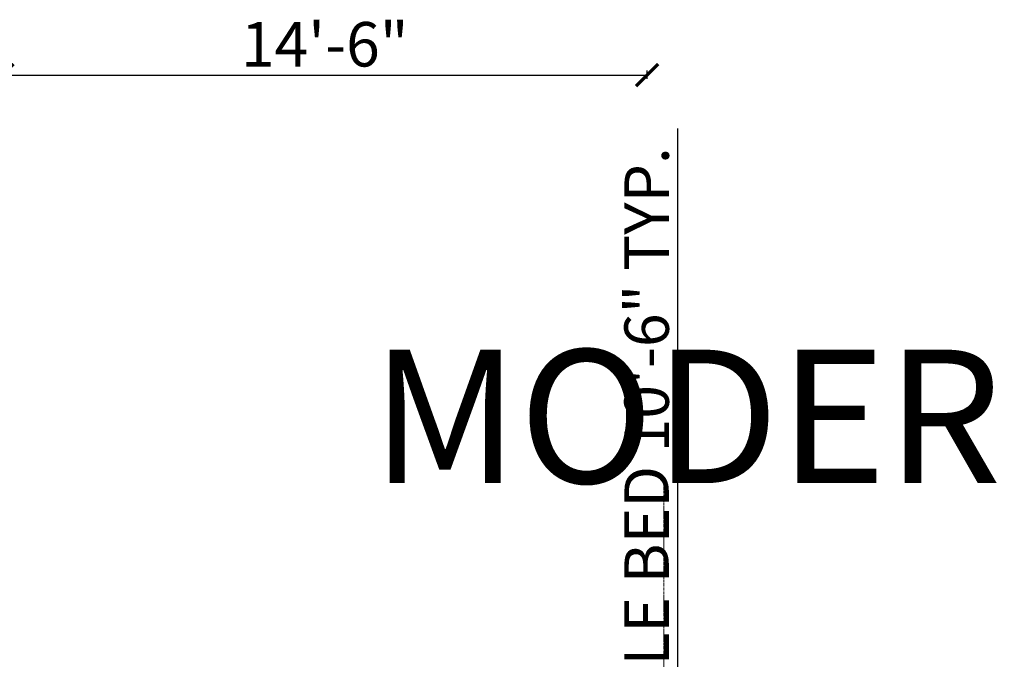
# Model space of a CAD drawing. Units: inches. Extents: x 261 to 2725, y 291 to 1454.
# Tile 16 of 35: x 777 to 1043, y 1281 to 1454. Entities that reach past the tile are written whole.
import ezdxf

# ---------------------------------------------------------------- set-up
doc = ezdxf.new("R2010")
doc.units = ezdxf.units.IN
doc.linetypes.add('CENTER', pattern=[2, 1.25, -0.25, 0.25, -0.25])
for name, color, linetype, lineweight in [('A-ANNO-DIMS', 136, 'Continuous', 18), ('A-ANNO-TEXT', 7, 'Continuous', 25), ('A-GRID', 251, 'CENTER', 13)]:
    doc.layers.add(name, color=color, linetype=linetype, lineweight=lineweight)
doc.styles.get("Standard").update_dxf_attribs({"font": 'arial.ttf'})
doc.dimstyles.new('ISO-25', dxfattribs={"dimtxt": 12, "dimasz": 6, "dimexe": 1.25, "dimexo": 0.625, "dimtad": 1, "dimdec": 0, "dimlunit": 3, "dimtxsty": 'Standard', "dimblk": 'ARCHTICK', "dimcen": 2.5, "dimadec": 0, "dimazin": 0, "dimtfac": 1, "dimtdec": 0, "dimtmove": 0, "dimatfit": 3, "dimfxl": 1, "dimfxlon": 1, "dimarcsym": 0})

# ---------------------------------------------------------------- blocks, each defined once
blk = doc.blocks.new('_ArchTick')
at = {"color": 0, "linetype": 'ByBlock', "const_width": 0.15}
blk.add_lwpolyline([(-0.5, -0.5), (0.5, 0.5)], dxfattribs=at)
blk = doc.blocks.new('*D41')
at = {"layer": 'A-ANNO-DIMS', "color": 0, "lineweight": -2, "ltscale": 0.07, "transparency": 16777216}
for p, q in [((954.74, 1222.47), (954.74, 1424.31)), ((953.74, 1222.47), (955.99, 1222.47)), ((954.74, 1096.37), (954.74, 1222.47)), ((953.74, 1096.37), (955.99, 1096.37))]:
    blk.add_line(p, q, dxfattribs=at)
at = {"layer": 'Defpoints', "color": 0, "ltscale": 0.07, "transparency": 16777216}
for p in [(935.82, 1222.47), (954.74, 1222.47), (935.82, 1096.37)]:
    blk.add_point(p, dxfattribs=at)
at = {"layer": 'A-ANNO-DIMS', "color": 0, "lineweight": -2, "ltscale": 0.07, "transparency": 16777216, "xscale": 6, "yscale": 6, "zscale": 6}
for p, rotation in [((954.74, 1222.47), 90), ((954.74, 1096.37), 270)]:
    blk.add_blockref('_ArchTick', p, dxfattribs=dict(at, rotation=rotation))
at = {"layer": 'A-ANNO-DIMS', "color": 0, "ltscale": 0.07, "transparency": 16777216, "insert": (947.9, 1326.39), "char_height": 12, "attachment_point": 5, "rotation": 90}
blk.add_mtext('DOUBLE BED 10\'-6" TYP.', dxfattribs=at)
blk = doc.blocks.new('*D76')
at = {"layer": 'A-ANNO-DIMS', "color": 0, "lineweight": -2, "ltscale": 0.07, "transparency": 16777216}
for p, q in [((772.45, 1437.76), (772.45, 1440.01)), ((772.45, 1438.76), (946.45, 1438.76)), ((946.45, 1437.76), (946.45, 1440.01))]:
    blk.add_line(p, q, dxfattribs=at)
at = {"layer": 'Defpoints', "color": 0, "ltscale": 0.07, "transparency": 16777216}
for p in [(946.45, 1438.76), (772.45, 1222.47), (946.45, 1222.47)]:
    blk.add_point(p, dxfattribs=at)
at = {"layer": 'A-ANNO-DIMS', "color": 0, "lineweight": -2, "ltscale": 0.07, "transparency": 16777216, "xscale": 6, "yscale": 6, "zscale": 6, "rotation": 180}
blk.add_blockref('_ArchTick', (772.45, 1438.76), dxfattribs=at)
at = {"layer": 'A-ANNO-DIMS', "color": 0, "lineweight": -2, "ltscale": 0.07, "transparency": 16777216, "xscale": 6, "yscale": 6, "zscale": 6}
blk.add_blockref('_ArchTick', (946.45, 1438.76), dxfattribs=at)
at = {"layer": 'A-ANNO-DIMS', "color": 0, "ltscale": 0.07, "transparency": 16777216, "insert": (859.45, 1445.51), "char_height": 12, "attachment_point": 5}
blk.add_mtext('14\'-6"', dxfattribs=at)

msp = doc.modelspace()

# ---------------------------------------------------------------- linework, layer by layer
at = {"layer": 'A-GRID', "ltscale": 0.5}
msp.add_line((950.95, 1330.47), (950.95, 416.47), dxfattribs=at)

# ---------------------------------------------------------------- texts
at = {"layer": 'A-ANNO-TEXT', "insert": (872, 1364.68), "char_height": 36, "attachment_point": 1}
msp.add_mtext_dynamic_manual_height_columns('{\\fTimes New Roman|b1|i0|c0|p18;\\T1.4;MODERN MANSION 2D DESIGNS}', width=1067.3388, gutter_width=12.5, heights=[0], dxfattribs=at)

# ---------------------------------------------------------------- dimensions: what is measured, and where the dimension line sits
at = {"layer": 'A-ANNO-DIMS', "ltscale": 0.07}
dim = msp.add_linear_dim(base=(946.45, 1438.76), p1=(772.45, 1222.47), p2=(946.45, 1222.47), dimstyle='ISO-25', override={"dimdec": 1, "dimlfac": 1, "dimrnd": 0, "dimzin": 1, "dimdsep": 46, "dimlunit": 4, "dimfrac": 2}, dxfattribs=at)
dim.commit()
dim.dimension.update_dxf_attribs({"geometry": '*D76', "text_midpoint": (859.45, 1445.51)})
dim = msp.add_linear_dim(base=(954.74, 1222.47), p1=(935.82, 1096.37), p2=(935.82, 1222.47), angle=90, text='DOUBLE BED <> TYP.', dimstyle='ISO-25', override={"dimdec": 1, "dimrnd": 0, "dimzin": 1, "dimlunit": 4, "dimfrac": 2}, dxfattribs=at)
dim.commit()
dim.dimension.update_dxf_attribs({"geometry": '*D41', "text_midpoint": (947.9, 1326.39)})

doc.saveas('drawing.dxf')
